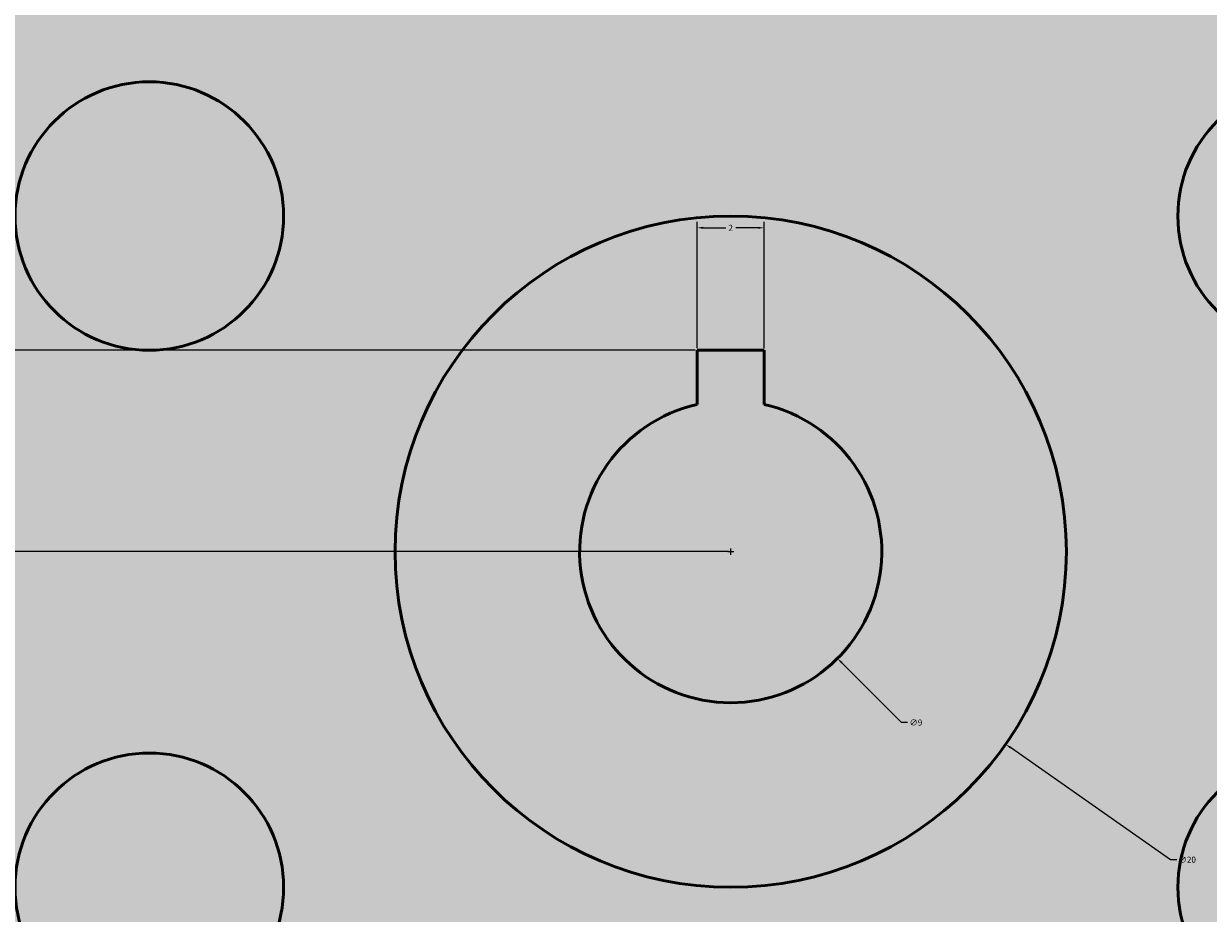
# Model space of a CAD drawing. Units: millimetres. Extents: x 2943.6 to 3032.7, y 1562 to 1639.7.
# Tile 5 of 9: x 2961.4 to 2996.7, y 1590.1 to 1616.6. Entities that reach past the tile are written whole.
import ezdxf

# ---------------------------------------------------------------- set-up
doc = ezdxf.new("R2010")
doc.units = ezdxf.units.MM
doc.layers.add('M-DIMS', color=2, linetype='Continuous', lineweight=18)
doc.layers.add('M-OUTL', color=7, linetype='Continuous', lineweight=50)
doc.layers.add('M-HATC', color=7, linetype='Continuous', lineweight=18, true_color=0xffffff)
doc.styles.get("Standard").update_dxf_attribs({"font": 'arial.ttf'})
doc.dimstyles.get("Standard").update_dxf_attribs({"dimtxt": 0.18, "dimasz": 0.18, "dimexe": 0.18, "dimexo": 0.0625, "dimgap": 0.09, "dimtad": 0, "dimtih": 1, "dimtoh": 1, "dimdec": 4, "dimzin": 0, "dimdsep": 46, "dimtxsty": 'Standard', "dimcen": 0.09, "dimadec": 0, "dimazin": 0, "dimtfac": 1, "dimtdec": 4, "dimtofl": 0, "dimtmove": 0, "dimatfit": 3, "dimfxl": 1, "dimtolj": 1, "dimtzin": 0, "dimarcsym": 0})

# ---------------------------------------------------------------- blocks, each defined once
blk = doc.blocks.new('*U1')
blk.add_circle((0, 0), 4)
blk = doc.blocks.new('*U2')
at = {"layer": 'M-OUTL', "color": 0, "linetype": 'ByBlock', "lineweight": -2, "transparency": 16777216}
for p, rotation in [((2965.149, 1610.848), 59.99999999999999), ((2999.79, 1610.848), 300), ((2965.149, 1590.848), 120), ((2999.79, 1590.848), 240)]:
    blk.add_blockref('*U1', p, dxfattribs=dict(at, rotation=rotation))
blk = doc.blocks.new('*D3')
at = {"layer": 'Defpoints', "color": 0, "transparency": 16777216}
for p in [(2947.469, 1600.848), (3017.469, 1600.848), (3017.469, 1562.198)]:
    blk.add_point(p, dxfattribs=at)
at = {"layer": 'M-DIMS', "color": 0, "lineweight": -2, "transparency": 16777216}
for p, q in [((2947.469, 1600.786), (2947.469, 1562.018)), ((3017.469, 1600.786), (3017.469, 1562.018)), ((2947.649, 1562.198), (2982.251, 1562.198)), ((3017.289, 1562.198), (2982.687, 1562.198))]:
    blk.add_line(p, q, dxfattribs=at)
at = {"layer": 'M-DIMS', "color": 0, "transparency": 16777216}
for points in [[(2947.649, 1562.228), (2947.649, 1562.168), (2947.469, 1562.198)], [(3017.289, 1562.228), (3017.289, 1562.168), (3017.469, 1562.198)]]:
    blk.add_solid(points, dxfattribs=at)
at = {"layer": 'M-DIMS', "color": 0, "transparency": 16777216, "insert": (2982.469, 1562.198), "char_height": 0.18, "attachment_point": 5}
blk.add_mtext('\\A1;70', dxfattribs=at)
blk = doc.blocks.new('*D4')
at = {"layer": 'Defpoints', "color": 0, "transparency": 16777216}
for p in [(2943.819, 1635.848), (2982.469, 1635.848), (2982.469, 1565.848)]:
    blk.add_point(p, dxfattribs=at)
at = {"layer": 'M-DIMS', "color": 0, "lineweight": -2, "transparency": 16777216}
for p, q in [((2982.407, 1635.848), (2943.639, 1635.848)), ((2943.819, 1635.668), (2943.819, 1601.03)), ((2943.819, 1566.028), (2943.819, 1600.666)), ((2982.407, 1565.848), (2943.639, 1565.848))]:
    blk.add_line(p, q, dxfattribs=at)
at = {"layer": 'M-DIMS', "color": 0, "transparency": 16777216}
for points in [[(2943.789, 1635.668), (2943.849, 1635.668), (2943.819, 1635.848)], [(2943.789, 1566.028), (2943.849, 1566.028), (2943.819, 1565.848)]]:
    blk.add_solid(points, dxfattribs=at)
at = {"layer": 'M-DIMS', "color": 0, "transparency": 16777216, "insert": (2943.819, 1600.848), "char_height": 0.18, "attachment_point": 5}
blk.add_mtext('\\A1;70', dxfattribs=at)
blk = doc.blocks.new('*D5')
at = {"layer": 'Defpoints', "color": 0, "transparency": 16777216}
for p in [(2986.469, 1620.848), (3021.119, 1620.848), (2986.469, 1580.848)]:
    blk.add_point(p, dxfattribs=at)
at = {"layer": 'M-DIMS', "color": 0, "lineweight": -2, "transparency": 16777216}
for p, q in [((2986.532, 1620.848), (3021.299, 1620.848)), ((3021.119, 1620.668), (3021.119, 1601.03)), ((3021.119, 1581.028), (3021.119, 1600.666)), ((2986.532, 1580.848), (3021.299, 1580.848))]:
    blk.add_line(p, q, dxfattribs=at)
at = {"layer": 'M-DIMS', "color": 0, "transparency": 16777216}
for points in [[(3021.089, 1620.668), (3021.149, 1620.668), (3021.119, 1620.848)], [(3021.089, 1581.028), (3021.149, 1581.028), (3021.119, 1580.848)]]:
    blk.add_solid(points, dxfattribs=at)
at = {"layer": 'M-DIMS', "color": 0, "transparency": 16777216, "insert": (3021.119, 1600.848), "char_height": 0.18, "attachment_point": 5}
blk.add_mtext('\\A1;40', dxfattribs=at)
blk = doc.blocks.new('*D8')
at = {"layer": 'Defpoints', "color": 0, "transparency": 16777216}
for p in [(2983.469, 1610.498), (2981.469, 1606.848), (2983.469, 1606.848)]:
    blk.add_point(p, dxfattribs=at)
at = {"layer": 'M-DIMS', "color": 0, "lineweight": -2, "transparency": 16777216}
for p, q in [((2981.469, 1606.911), (2981.469, 1610.678)), ((2983.469, 1606.911), (2983.469, 1610.678)), ((2981.649, 1610.498), (2982.32, 1610.498)), ((2983.289, 1610.498), (2982.619, 1610.498))]:
    blk.add_line(p, q, dxfattribs=at)
at = {"layer": 'M-DIMS', "color": 0, "transparency": 16777216}
for points in [[(2981.649, 1610.528), (2981.649, 1610.468), (2981.469, 1610.498)], [(2983.289, 1610.528), (2983.289, 1610.468), (2983.469, 1610.498)]]:
    blk.add_solid(points, dxfattribs=at)
at = {"layer": 'M-DIMS', "color": 0, "transparency": 16777216, "insert": (2982.469, 1610.498), "char_height": 0.18, "attachment_point": 5}
blk.add_mtext('\\A1;2', dxfattribs=at)
blk = doc.blocks.new('*D9')
at = {"layer": 'Defpoints', "color": 0, "transparency": 16777216}
for p in [(2943.819, 1606.848), (2981.469, 1606.848), (2982.469, 1600.848)]:
    blk.add_point(p, dxfattribs=at)
at = {"layer": 'M-DIMS', "color": 0, "lineweight": -2, "transparency": 16777216}
for p, q in [((2981.407, 1606.848), (2943.639, 1606.848)), ((2943.819, 1606.668), (2943.819, 1604.03)), ((2943.819, 1601.028), (2943.819, 1603.666)), ((2982.407, 1600.848), (2943.639, 1600.848))]:
    blk.add_line(p, q, dxfattribs=at)
at = {"layer": 'M-DIMS', "color": 0, "transparency": 16777216}
for points in [[(2943.789, 1606.668), (2943.849, 1606.668), (2943.819, 1606.848)], [(2943.789, 1601.028), (2943.849, 1601.028), (2943.819, 1600.848)]]:
    blk.add_solid(points, dxfattribs=at)
at = {"layer": 'M-DIMS', "color": 0, "transparency": 16777216, "insert": (2943.819, 1603.848), "char_height": 0.18, "attachment_point": 5}
blk.add_mtext('\\A1;6', dxfattribs=at)
blk = doc.blocks.new('*D10')
at = {"layer": 'Defpoints', "color": 0, "transparency": 16777216}
for p in [(3013.14, 1615.522), (2982.469, 1600.848)]:
    blk.add_point(p, dxfattribs=at)
at = {"layer": 'M-DIMS', "color": 0, "lineweight": -2, "transparency": 16777216}
for p, q in [((3031.542, 1624.326), (3013.302, 1615.6)), ((3031.722, 1624.326), (3031.542, 1624.326)), ((2982.379, 1600.848), (2982.559, 1600.848)), ((2982.469, 1600.758), (2982.469, 1600.938))]:
    blk.add_line(p, q, dxfattribs=at)
at = {"layer": 'M-DIMS', "color": 0, "transparency": 16777216}
blk.add_solid([(3013.289, 1615.627), (3013.315, 1615.573), (3013.14, 1615.522)], dxfattribs=at)
at = {"layer": 'M-DIMS', "color": 0, "transparency": 16777216, "insert": (3032.292, 1624.326), "char_height": 0.18, "attachment_point": 5}
blk.add_mtext('\\A1;28X R34', dxfattribs=at)
blk = doc.blocks.new('*D11')
at = {"layer": 'Defpoints', "color": 0, "transparency": 16777216}
for p in [(2974.278, 1606.585), (2990.66, 1595.112)]:
    blk.add_point(p, dxfattribs=at)
at = {"layer": 'M-DIMS', "color": 0, "lineweight": -2, "transparency": 16777216}
for p, q in [((2982.379, 1600.848), (2982.559, 1600.848)), ((2982.469, 1600.758), (2982.469, 1600.938)), ((2995.575, 1591.67), (2990.808, 1595.009)), ((2995.755, 1591.67), (2995.575, 1591.67))]:
    blk.add_line(p, q, dxfattribs=at)
at = {"layer": 'M-DIMS', "color": 0, "transparency": 16777216}
blk.add_solid([(2990.825, 1595.033), (2990.791, 1594.984), (2990.66, 1595.112)], dxfattribs=at)
at = {"layer": 'M-DIMS', "color": 0, "transparency": 16777216, "insert": (2996.071, 1591.67), "char_height": 0.18, "attachment_point": 5}
blk.add_mtext('\\A1;∅20', dxfattribs=at)
blk = doc.blocks.new('*D12')
at = {"layer": 'Defpoints', "color": 0, "transparency": 16777216}
for p in [(2979.288, 1604.031), (2985.651, 1597.666)]:
    blk.add_point(p, dxfattribs=at)
at = {"layer": 'M-DIMS', "color": 0, "lineweight": -2, "transparency": 16777216}
for p, q in [((2982.379, 1600.848), (2982.559, 1600.848)), ((2982.469, 1600.758), (2982.469, 1600.938)), ((2987.56, 1595.757), (2985.778, 1597.539)), ((2987.74, 1595.757), (2987.56, 1595.757))]:
    blk.add_line(p, q, dxfattribs=at)
at = {"layer": 'M-DIMS', "color": 0, "transparency": 16777216}
blk.add_solid([(2985.799, 1597.56), (2985.757, 1597.518), (2985.651, 1597.666)], dxfattribs=at)
at = {"layer": 'M-DIMS', "color": 0, "transparency": 16777216, "insert": (2987.987, 1595.757), "char_height": 0.18, "attachment_point": 5}
blk.add_mtext('\\A1;∅9', dxfattribs=at)

msp = doc.modelspace()

# ---------------------------------------------------------------- hatches: boundary and pattern name
at = {"layer": 'M-HATC'}
h = msp.add_hatch(color=256, dxfattribs=at)
h.set_gradient(color1=(0, 0, 255), color2=(255, 255, 0), tint=1, name='INVCURVED')
h.paths.add_polyline_path([(2949.361, 1608.583, 0.001279), (2949.322, 1608.414), (2948.347, 1608.637), (2948.473, 1600.848), (2947.469, 1600.848), (2949.283, 1593.452, 0.001279), (2949.322, 1593.283), (2948.347, 1593.06), (2951.761, 1586.253, 0.001279), (2951.836, 1586.096), (2950.935, 1585.662), (2955.779, 1579.786, 0.001279), (2955.887, 1579.65), (2955.105, 1579.026), (2961.135, 1574.375, 0.001279), (2961.271, 1574.266), (2960.647, 1573.484), (2967.561, 1570.291, 0.001279), (2967.717, 1570.215), (2967.283, 1569.314), (2974.734, 1567.74, 0.001279), (2974.904, 1567.701), (2974.681, 1566.726), (2982.295, 1566.849, 0.001279), (2982.469, 1566.848), (2982.469, 1565.848), (2989.865, 1567.662, 0.001279), (2990.035, 1567.701), (2990.258, 1566.726), (2997.064, 1570.14, 0.001279), (2997.221, 1570.215), (2997.655, 1569.314), (3003.532, 1574.158, 0.001279), (3003.668, 1574.266), (3004.291, 1573.484), (3008.943, 1579.514, 0.001279), (3009.052, 1579.65), (3009.833, 1579.026), (3013.026, 1585.94, 0.001279), (3013.102, 1586.096), (3014.003, 1585.662), (3015.578, 1593.113, 0.001279), (3015.617, 1593.283), (3016.592, 1593.06), (3016.469, 1600.674, 0.001279), (3016.469, 1600.848), (3017.469, 1600.848), (3015.655, 1608.244, 0.001279), (3015.617, 1608.414), (3016.592, 1608.637), (3013.177, 1615.443, 0.001279), (3013.102, 1615.6), (3014.003, 1616.034), (3009.16, 1621.911, 0.001279), (3009.052, 1622.047), (3009.833, 1622.67), (3003.804, 1627.322, 0.001279), (3003.668, 1627.431), (3004.291, 1628.212), (2997.378, 1631.405, 0.001279), (2997.221, 1631.481), (2997.655, 1632.382), (2990.204, 1633.957, 0.001279), (2990.035, 1633.996), (2990.258, 1634.971), (2982.469, 1634.845), (2982.469, 1635.848), (2975.073, 1634.034, 0.001279), (2974.904, 1633.996), (2974.681, 1634.971), (2967.874, 1631.556, 0.001279), (2967.717, 1631.481), (2967.283, 1632.382), (2961.407, 1627.539, 0.001279), (2961.271, 1627.431), (2960.647, 1628.212), (2955.996, 1622.183, 0.001279), (2955.887, 1622.047), (2955.105, 1622.67), (2951.912, 1615.757, 0.001279), (2951.836, 1615.6), (2950.935, 1616.034)])
h.paths.add_polyline_path([(2969.149, 1610.848, -1), (2961.149, 1610.848, -1)], flags=16)
h.paths.add_polyline_path([(2969.149, 1590.848, -1), (2961.149, 1590.848, -1)], flags=16)
h.paths.add_polyline_path([(2992.469, 1600.848, -1), (2972.469, 1600.848, -1)], flags=16)
h.paths.add_polyline_path([(2978.469, 1620.848, -1), (2986.469, 1620.848, -1)], flags=16)
h.paths.add_polyline_path([(2981.469, 1605.236), (2981.469, 1606.848), (2983.469, 1606.848), (2983.469, 1605.236, -8.887482)], flags=0)
h.paths.add_polyline_path([(2986.469, 1580.848, -1), (2978.469, 1580.848, -1)], flags=16)
h.paths.add_polyline_path([(3003.79, 1610.848, -1), (2995.79, 1610.848, -1)], flags=16)
h.paths.add_polyline_path([(3003.79, 1590.848, -1), (2995.79, 1590.848, -1)], flags=16)
h = msp.add_hatch(color=256, dxfattribs=at)
h.paths.add_polyline_path([(2978.469, 1620.848, 1), (2986.469, 1620.848, 1)])
h.paths.add_polyline_path([(2995.79, 1610.848, 1), (3003.79, 1610.848, 1)])
h.paths.add_polyline_path([(3003.79, 1590.848, 1), (2995.79, 1590.848, 1)])
h.paths.add_polyline_path([(2986.469, 1580.848, 1), (2978.469, 1580.848, 1)])
h.paths.add_polyline_path([(2969.149, 1590.848, 1), (2961.149, 1590.848, 1)])
h.paths.add_polyline_path([(2961.149, 1610.848, 1), (2969.149, 1610.848, 1)])
h = msp.add_hatch(color=256, dxfattribs=at)
h.set_gradient(color1=(0, 0, 255), color2=(255, 255, 0), name='INVSPHERICAL')
h.paths.add_polyline_path([(2992.469, 1600.848, 1), (2972.469, 1600.848, 1)])
h.paths.add_polyline_path([(2981.469, 1605.236), (2981.469, 1606.848), (2983.469, 1606.848), (2983.469, 1605.236, -8.887482)], flags=16)
h = msp.add_hatch(color=256, dxfattribs=at)
h.set_gradient(color1=(0, 0, 255), color2=(255, 255, 0), tint=1)
h.paths.add_polyline_path([(2983.469, 1605.236), (2983.469, 1606.848), (2981.469, 1606.848), (2981.469, 1605.236, 8.887482)])

# ---------------------------------------------------------------- linework, layer by layer
at = {"layer": 'M-OUTL'}
for p, q in [((2981.469, 1606.848), (2983.469, 1606.848)), ((2981.469, 1605.236), (2981.469, 1606.848)), ((2983.469, 1605.236), (2983.469, 1606.848))]:
    msp.add_line(p, q, dxfattribs=at)
msp.add_circle((2982.469, 1600.848), 10, dxfattribs=at)
msp.add_arc((2982.469, 1600.848), 4.5, 102.8396, 77.1604, dxfattribs=at)

# ---------------------------------------------------------------- block references
msp.add_blockref('*U2', (0, 0), dxfattribs=at)

# ---------------------------------------------------------------- dimensions: what is measured, and where the dimension line sits
at = {"layer": 'M-DIMS'}
for base, p1, p2, picture, middle in [((2943.819, 1635.848), (2982.469, 1565.848), (2982.469, 1635.848), '*D4', (2943.819, 1600.848)), ((3021.119, 1620.848), (2986.469, 1580.848), (2986.469, 1620.848), '*D5', (3021.119, 1600.848)), ((2943.819, 1606.848), (2982.469, 1600.848), (2981.469, 1606.848), '*D9', (2943.819, 1603.848))]:
    dim = msp.add_linear_dim(base=base, p1=p1, p2=p2, angle=90, dimstyle='Standard', override={"dimdec": 0, "dimlfac": 1, "dimrnd": 0, "dimzin": 0, "dimdsep": 46, "dimlunit": 2}, dxfattribs=at)
    dim.commit()
    dim.dimension.update_dxf_attribs({"geometry": picture, "text_midpoint": middle})
dim = msp.add_radius_dim(center=(2982.469, 1600.848), mpoint=(3013.14, 1615.522), text='28X <>', dimstyle='Standard', override={"dimdec": 0, "dimlfac": 1, "dimrnd": 0, "dimzin": 0, "dimdsep": 46, "dimlunit": 2}, dxfattribs=at)
dim.commit()
dim.dimension.update_dxf_attribs({"geometry": '*D10', "text_midpoint": (3032.292, 1624.326), "dimtype": 164})
for base, p1, p2, picture, middle in [((2983.469, 1610.498), (2981.469, 1606.848), (2983.469, 1606.848), '*D8', (2982.469, 1610.498)), ((3017.469, 1562.198), (2947.469, 1600.848), (3017.469, 1600.848), '*D3', (2982.469, 1562.198))]:
    dim = msp.add_linear_dim(base=base, p1=p1, p2=p2, dimstyle='Standard', override={"dimdec": 0, "dimlfac": 1, "dimrnd": 0, "dimzin": 0, "dimdsep": 46, "dimlunit": 2}, dxfattribs=at)
    dim.commit()
    dim.dimension.update_dxf_attribs({"geometry": picture, "text_midpoint": middle})
for p1, p2, picture, middle in [((2974.278, 1606.585), (2990.66, 1595.112), '*D11', (2996.071, 1591.67)), ((2979.288, 1604.031), (2985.651, 1597.666), '*D12', (2987.987, 1595.757))]:
    dim = msp.add_diameter_dim_2p(p1=p1, p2=p2, dimstyle='Standard', override={"dimdec": 0, "dimlfac": 1, "dimrnd": 0, "dimzin": 0, "dimdsep": 46, "dimlunit": 2}, dxfattribs=at)
    dim.commit()
    dim.dimension.update_dxf_attribs({"geometry": picture, "text_midpoint": middle, "dimtype": 163})

doc.saveas('drawing.dxf')
